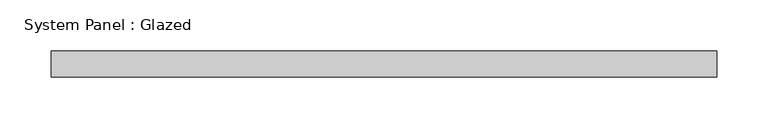
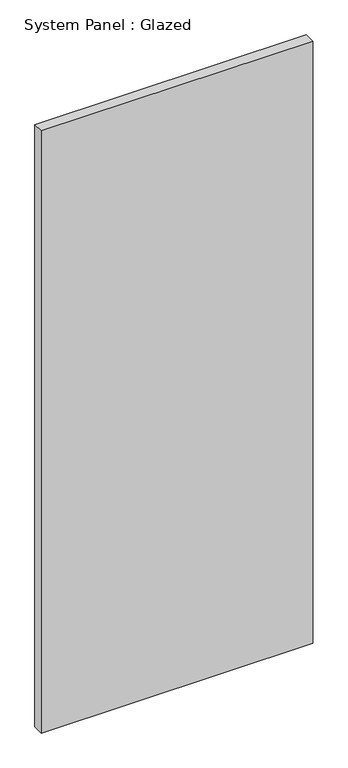
"""IFC4 building model written with IfcOpenShell, lengths in millimetres: plate geometry, System Panel : Glazed."""

from ifc_helpers import new_model, si_unit, origin, origin_with_axes, place, context, project, spatial, polyline, outline, extrude, source, transform, mapped, element, save


def system_panel_glazed_c581bff3(model_context):
    return source(origin(), model_context, "Body", "SweptSolid", [
        extrude(outline(polyline([(323.85, 19.05), (-323.85, 19.05), (-323.85, 44.45), (323.85, 44.45), (323.85, 19.05)])), origin_with_axes(), (0.0, 0.0, 1.0), 1518.4701172),
    ])


if __name__ == "__main__":
    model = new_model("IFC4")
    model_context = context("Model", 3, world=origin())
    ifc_project = project(units=[si_unit("LENGTHUNIT", "METRE", prefix="MILLI")], contexts=[model_context])
    site = spatial("IfcSite", under=ifc_project)
    building = spatial("IfcBuilding", under=site)
    placement = place(None, origin())
    system_panel_glazed_shape = system_panel_glazed_c581bff3(model_context)
    element("IfcPlate", 1, ObjectType="System Panel : Glazed", at=placement, inside=building, context=model_context, shape_type="MappedRepresentation", body=[
        mapped(system_panel_glazed_shape, transform((0.0, 0.0, 0.0), x_axis=(1.0, 0.0, 0.0), y_axis=(0.0, 1.0, 0.0), z_axis=(0.0, 0.0, 1.0))),
    ])
    save(model, "model.ifc")

# Revit data of these elements
# Type "System Panel : Glazed"
#   Construction Type Id = "GSP4R"
#   Analytic Construction = "1/8 in Pilkington single glazing"
#   Visual Light Transmittance = 0.9
#   Solar Heat Gain Coefficient = 0.86
#   Heat Transfer Coefficient (U) = 1.18115 BTU/(h·ft²·°F)
#   Define Thermal Properties by = 1
# Element 1 (IfcPlate, "System Panel : Glazed")
#   Materials on its faces: "Glass"
# Materials
#   "Glass": class "Glass", colour RGB 0 128 192, transparency 0.75, Description = "Soda Lime Glass", Cost = 0
